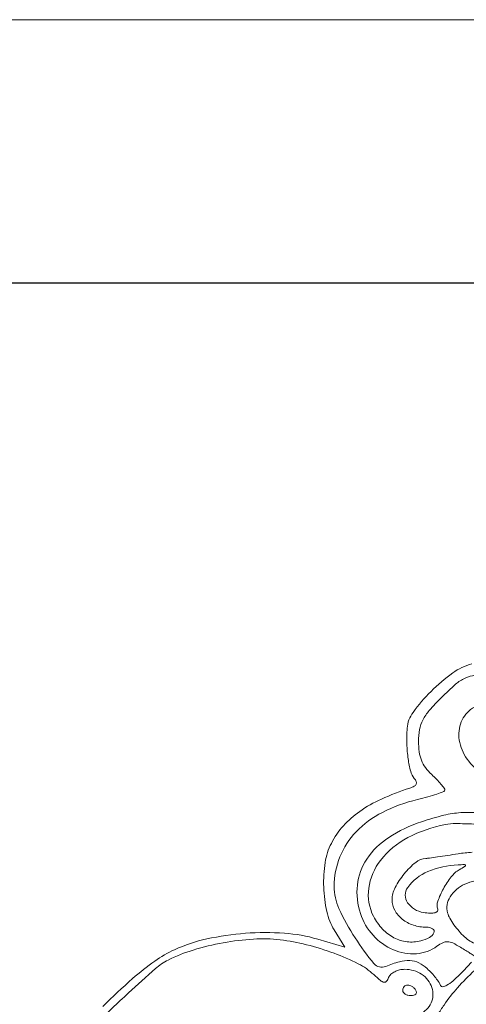
# Model space of a CAD drawing. Units: inches. Extents: x 2656 to 9931, y 1941 to 3068.
# Tile 39 of 46: x 2836.92 to 2842.88, y 2981.19 to 2994.35. Entities that reach past the tile are written whole.
import ezdxf

# ---------------------------------------------------------------- set-up
doc = ezdxf.new("R2010")
doc.units = ezdxf.units.IN
for name, color, linetype, lineweight in [('A-ANNO-DIMS', 2, 'Continuous', 18), ('A-ELEV-FNSH', 8, 'Continuous', 13), ('A-ELEV-ORN', 8, 'Continuous', 13)]:
    doc.layers.add(name, color=color, linetype=linetype, lineweight=lineweight)
doc.styles.get("Standard").update_dxf_attribs({"font": 'arial.ttf'})
doc.dimstyles.new('ISO-25', dxfattribs={"dimtxt": 6, "dimasz": 2.5, "dimexe": 1.25, "dimexo": 0.625, "dimtad": 1, "dimdec": 0, "dimlunit": 3, "dimtxsty": 'Standard', "dimcen": 2.5, "dimadec": 0, "dimazin": 0, "dimtfac": 1, "dimtdec": 0, "dimtmove": 0, "dimatfit": 3, "dimfxl": 1, "dimarcsym": 0})

# ---------------------------------------------------------------- blocks, each defined once
blk = doc.blocks.new('*D152')
at = {"layer": 'A-ANNO-DIMS', "color": 0, "lineweight": -2, "transparency": 16777216}
for p, q in [((2847.28, 2990.828), (2707.323, 2990.828)), ((2708.573, 2988.328), (2708.573, 2952.971)), ((2847.248, 2950.471), (2707.323, 2950.471))]:
    blk.add_line(p, q, dxfattribs=at)
at = {"layer": 'A-ANNO-DIMS', "color": 0, "transparency": 16777216}
for points in [[(2708.156, 2988.328), (2708.989, 2988.328), (2708.573, 2990.828)], [(2708.156, 2952.971), (2708.989, 2952.971), (2708.573, 2950.471)]]:
    blk.add_solid(points, dxfattribs=at)
at = {"layer": 'Defpoints', "color": 0, "transparency": 16777216}
for p in [(2847.905, 2990.828), (2708.573, 2950.471), (2847.873, 2950.471)]:
    blk.add_point(p, dxfattribs=at)
at = {"layer": 'A-ANNO-DIMS', "color": 0, "transparency": 16777216, "insert": (2704.843, 2970.649), "char_height": 6, "attachment_point": 5, "rotation": 90}
blk.add_mtext('3\'-4 1/2"', dxfattribs=at)
blk = doc.blocks.new('*D153')
at = {"layer": 'A-ANNO-DIMS', "color": 0, "lineweight": -2, "transparency": 16777216}
for p, q in [((2826.64, 2993.722), (2826.64, 2703.709)), ((2829.546, 2956.424), (2829.546, 2703.709)), ((2824.14, 2704.959), (2821.64, 2704.959)), ((2826.64, 2704.959), (2829.546, 2704.959)), ((2832.046, 2704.959), (2851.745, 2704.959))]:
    blk.add_line(p, q, dxfattribs=at)
at = {"layer": 'A-ANNO-DIMS', "color": 0, "transparency": 16777216}
for points in [[(2824.14, 2705.376), (2824.14, 2704.543), (2826.64, 2704.959)], [(2832.046, 2705.376), (2832.046, 2704.543), (2829.546, 2704.959)]]:
    blk.add_solid(points, dxfattribs=at)
at = {"layer": 'Defpoints', "color": 0, "transparency": 16777216}
for p in [(2826.64, 2994.347), (2829.546, 2957.049), (2829.546, 2704.959)]:
    blk.add_point(p, dxfattribs=at)
at = {"layer": 'A-ANNO-DIMS', "color": 0, "transparency": 16777216, "insert": (2843.145, 2708.65), "char_height": 6, "attachment_point": 5}
blk.add_mtext('0\'-3"', dxfattribs=at)
blk = doc.blocks.new('*D154')
at = {"layer": 'A-ANNO-DIMS', "color": 0, "lineweight": -2, "transparency": 16777216}
for p, q in [((2708.573, 2996.847), (2708.573, 2999.347)), ((2826.015, 2994.347), (2707.323, 2994.347)), ((2708.573, 2994.347), (2708.573, 2990.828)), ((2847.28, 2990.828), (2707.323, 2990.828)), ((2708.573, 2988.328), (2708.573, 2954.647))]:
    blk.add_line(p, q, dxfattribs=at)
at = {"layer": 'A-ANNO-DIMS', "color": 0, "transparency": 16777216}
for points in [[(2708.156, 2996.847), (2708.989, 2996.847), (2708.573, 2994.347)], [(2708.156, 2988.328), (2708.989, 2988.328), (2708.573, 2990.828)]]:
    blk.add_solid(points, dxfattribs=at)
at = {"layer": 'Defpoints', "color": 0, "transparency": 16777216}
for p in [(2826.64, 2994.347), (2708.573, 2990.828), (2847.905, 2990.828)]:
    blk.add_point(p, dxfattribs=at)
at = {"layer": 'A-ANNO-DIMS', "color": 0, "transparency": 16777216, "insert": (2704.843, 2970.237), "char_height": 6, "attachment_point": 5, "rotation": 90}
blk.add_mtext('0\'-3 1/2"', dxfattribs=at)

msp = doc.modelspace()

# ---------------------------------------------------------------- linework, layer by layer
at = {"layer": 'A-ELEV-FNSH'}
msp.add_lwpolyline([(2826.64, 2994.347), (2868.226, 2994.347), (2868.226, 2892.035), (2826.64, 2892.035)], close=True, dxfattribs=at)
at = {"layer": 'A-ELEV-ORN'}
for points in [[(2842.958, 2985.742, 0.091949), (2842.702, 2985.62, 0.038622), (2842.412, 2985.372, 0.037417), (2842.171, 2985.093, 0.143658), (2842.093, 2984.88, 0.023892), (2842.089, 2984.669, 0.028098), (2842.106, 2984.47, 0.029751), (2842.14, 2984.305, 0.10751), (2842.188, 2984.211, -0.073762), (2842.214, 2984.168, -0.208767), (2842.213, 2984.134, -0.164765), (2842.187, 2984.106, -0.043658), (2842.129, 2984.081, 0.026739), (2841.749, 2983.935, 0.04806), (2841.459, 2983.769, 0.057169), (2841.241, 2983.576, 0.063024), (2841.081, 2983.343, 0.082479), (2840.998, 2983.088, 0.045446), (2840.979, 2982.758, 0.045504), (2841.02, 2982.432, 0.084728), (2841.12, 2982.186), (2841.262, 2981.956), (2840.899, 2982.063, 0.054117), (2840.454, 2982.142, 0.035583), (2839.934, 2982.141, 0.035558), (2839.418, 2982.066, 0.053588), (2838.988, 2981.922, 0.047177), (2838.723, 2981.769, 0.0258), (2838.429, 2981.536, 0.015337), (2838.032, 2981.164, 0.003566)], [(2842.951, 2981.755, -0.011717), (2842.882, 2981.678, -0.006865), (2842.795, 2981.589, -0.020091), (2842.701, 2981.502, -0.047456), (2842.623, 2981.447, -0.086049), (2842.567, 2981.427, -0.371007), (2842.539, 2981.444, 0.069167), (2842.518, 2981.485, 0.018604), (2842.475, 2981.544, 0.018474), (2842.42, 2981.609, 0.018164), (2842.36, 2981.669, 0.073955), (2842.248, 2981.746, 0.101291), (2842.13, 2981.777, 0.080634), (2841.99, 2981.761, 0.032402), (2841.807, 2981.698, -0.330166), (2841.65, 2981.736, -0.030568), (2841.399, 2982.079, -0.035399), (2841.183, 2982.472, -0.107926), (2841.119, 2982.768, -0.096197), (2841.195, 2983.161, -0.095451), (2841.412, 2983.497, -0.084847), (2841.764, 2983.757, -0.058752), (2842.23, 2983.928, 0.01005), (2842.37, 2983.964, 0.016008), (2842.488, 2984.001, 0.009984), (2842.582, 2984.036, 0.307534), (2842.596, 2984.056, 0.165147), (2842.588, 2984.08, 0.012602), (2842.544, 2984.134, 0.016249), (2842.487, 2984.196, 0.011634), (2842.42, 2984.263, -0.045336), (2842.337, 2984.356, -0.064574), (2842.283, 2984.453, -0.060363), (2842.254, 2984.565, -0.034085), (2842.244, 2984.706, -0.043672), (2842.258, 2984.865, -0.077311), (2842.301, 2984.99, -0.059), (2842.387, 2985.116, -0.016618), (2842.551, 2985.292, -0.01592), (2842.74, 2985.469, -0.072133), (2842.866, 2985.551, -0.083292), (2843.002, 2985.588, -0.025328)], [(2843.08, 2983.751, 0.032074), (2842.808, 2983.753, 0.046774), (2842.583, 2983.718, 0.018964), (2842.286, 2983.632, 0.062902), (2841.847, 2983.421, 0.103204), (2841.554, 2983.133, 0.120241), (2841.428, 2982.786, 0.107162), (2841.469, 2982.404, 0.105287), (2841.638, 2982.114, 0.10802), (2841.909, 2981.921, 0.117477), (2842.217, 2981.869, 0.142354), (2842.491, 2981.969, -0.04457), (2842.57, 2982.016, -0.12505), (2842.633, 2982.029, -0.103429), (2842.701, 2982.012, -0.025166), (2842.804, 2981.955, 0.000076), (2842.874, 2981.911, 0.000108), (2842.936, 2981.873, 0.000061), (2842.989, 2981.84, 0.001532)], [(2842.96, 2983.223, 0.031038), (2842.772, 2983.203, -0.002177), (2842.631, 2983.181, -0.002698), (2842.5, 2983.161, -0.002209), (2842.39, 2983.146, -0.020165), (2842.342, 2983.141, 0.157705), (2842.207, 2983.089, 0.051941), (2842.054, 2982.937, 0.051876), (2841.932, 2982.751, 0.119638), (2841.892, 2982.589, 0.124142), (2841.928, 2982.449, 0.101536), (2842.027, 2982.33, 0.090907), (2842.176, 2982.25, 0.077497), (2842.353, 2982.223, -0.135204), (2842.433, 2982.201, -0.37616), (2842.45, 2982.149, -0.169371), (2842.391, 2982.085, -0.062047), (2842.274, 2982.04, -0.090848), (2842.091, 2982.028, -0.0913), (2841.917, 2982.081, -0.08545), (2841.764, 2982.198, -0.068078), (2841.644, 2982.368, -0.155251), (2841.58, 2982.744, -0.13208), (2841.738, 2983.116, -0.10599), (2842.1, 2983.419, -0.074853), (2842.603, 2983.594, -0.047084), (2842.742, 2983.607, -0.010086), (2842.983, 2983.601, -0.010454)], [(2837.941, 2980.932, -0.007752), (2838.373, 2981.344, -0.006437), (2838.734, 2981.669, -0.063652), (2838.903, 2981.784, -0.042818), (2839.238, 2981.918, -0.028984), (2839.638, 2982.014, -0.029083), (2840.043, 2982.064, -0.045046), (2840.396, 2982.054, -0.03279), (2840.75, 2981.989, -0.026972), (2841.118, 2981.874, -0.027596), (2841.44, 2981.734, -0.072091), (2841.647, 2981.589, 0.014298), (2841.737, 2981.51, 0.127528), (2841.784, 2981.487, 0.279617), (2841.817, 2981.5, 0.075996), (2841.846, 2981.551, -0.118954), (2841.875, 2981.593, -0.06518), (2841.927, 2981.628, -0.059207), (2841.992, 2981.652, -0.05854), (2842.061, 2981.66, -0.146541), (2842.286, 2981.593, -0.167672), (2842.423, 2981.415, -0.192377), (2842.412, 2981.21, -0.182333), (2842.262, 2981.063, 0.022825)], [(2842.499, 2981.055, 0.000135), (2842.586, 2981.183, -0.032972), (2842.766, 2981.414, -0.024978), (2842.99, 2981.643, -0.020758)]]:
    msp.add_lwpolyline(points, format="xyb", dxfattribs=at)
for points in [[(2842.99, 2985.163, 0.150682), (2842.828, 2984.993, 0.140741), (2842.784, 2984.756, 0.118986), (2842.873, 2984.5, 0.09113), (2843.076, 2984.283, 0.047148), (2843.466, 2984.047, 0.03133), (2843.951, 2983.851, 0.029184), (2844.412, 2983.726, 0.144139), (2844.677, 2983.747, 0.505083), (2844.694, 2983.808, 0.008532), (2844.437, 2984.124, 0.014242), (2844.098, 2984.503, 0.008445), (2843.673, 2984.937, 0.045857), (2843.491, 2985.087, 0.069431), (2843.308, 2985.177, 0.084935), (2843.137, 2985.203, 0.123164)], [(2842.789, 2982.991, 0.095695), (2842.682, 2982.897, 0.040767), (2842.576, 2982.737, 0.039046), (2842.502, 2982.569, 0.173914), (2842.502, 2982.463, -0.274816), (2842.496, 2982.435, -0.155746), (2842.465, 2982.416, -0.069781), (2842.402, 2982.41, -0.023288), (2842.311, 2982.419, -0.205397), (2842.099, 2982.55, -0.320879), (2842.1, 2982.755, -0.14068), (2842.37, 2982.966, -0.083105), (2842.772, 2983.055, -0.005547), (2842.859, 2983.059, -0.346536), (2842.871, 2983.05, -0.333901), (2842.865, 2983.036, -0.00536)], [(2843.39, 2982.768, -0.122481), (2843.49, 2982.647, -0.068858), (2843.547, 2982.464, -0.069741), (2843.553, 2982.276, -0.137892), (2843.497, 2982.139, -0.099844), (2843.36, 2982.02, -0.111741), (2843.192, 2981.97, -0.109476), (2843.017, 2981.996, -0.092694), (2842.858, 2982.095, -0.030108), (2842.785, 2982.169, -0.024708), (2842.717, 2982.256, -0.025392), (2842.663, 2982.342, -0.058376), (2842.633, 2982.413, -0.219842), (2842.666, 2982.628, -0.137448), (2842.863, 2982.797, -0.118866), (2843.143, 2982.855, -0.152619)], [(2842.033, 2981.379, 0.153634), (2842.042, 2981.352, 0.097988), (2842.065, 2981.329, 0.080552), (2842.101, 2981.314, 0.062283), (2842.143, 2981.309, 0.066118), (2842.182, 2981.314, 0.138808), (2842.207, 2981.329, 0.191142), (2842.217, 2981.352, 0.139169), (2842.209, 2981.379, 0.06081), (2842.187, 2981.406, 0.051032), (2842.159, 2981.429, 0.053229), (2842.128, 2981.444, 0.089642), (2842.099, 2981.449, 0.105429), (2842.074, 2981.444, 0.099231), (2842.053, 2981.429, 0.096318), (2842.038, 2981.406, 0.092995)]]:
    msp.add_lwpolyline(points, format="xyb", close=True, dxfattribs=at)

# ---------------------------------------------------------------- dimensions: what is measured, and where the dimension line sits
at = {"layer": 'A-ANNO-DIMS'}
for base, p1, p2, picture, middle in [((2708.573, 2990.828), (2826.64, 2994.347), (2847.905, 2990.828), '*D154', (2704.843, 2970.237)), ((2708.573, 2950.471), (2847.905, 2990.828), (2847.873, 2950.471), '*D152', (2704.843, 2970.649))]:
    dim = msp.add_linear_dim(base=base, p1=p1, p2=p2, angle=90, dimstyle='ISO-25', override={"dimdec": 1, "dimlfac": 1, "dimrnd": 0, "dimzin": 1, "dimdsep": 46, "dimlunit": 4, "dimfrac": 2}, dxfattribs=at)
    dim.commit()
    dim.dimension.update_dxf_attribs({"geometry": picture, "text_midpoint": middle})
dim = msp.add_linear_dim(base=(2829.546, 2704.959), p1=(2826.64, 2994.347), p2=(2829.546, 2957.049), dimstyle='ISO-25', override={"dimdec": 1, "dimlfac": 1, "dimrnd": 0, "dimzin": 1, "dimdsep": 46, "dimlunit": 4, "dimfrac": 2}, dxfattribs=at)
dim.commit()
dim.dimension.update_dxf_attribs({"geometry": '*D153', "text_midpoint": (2843.145, 2708.65)})

doc.saveas('drawing.dxf')
